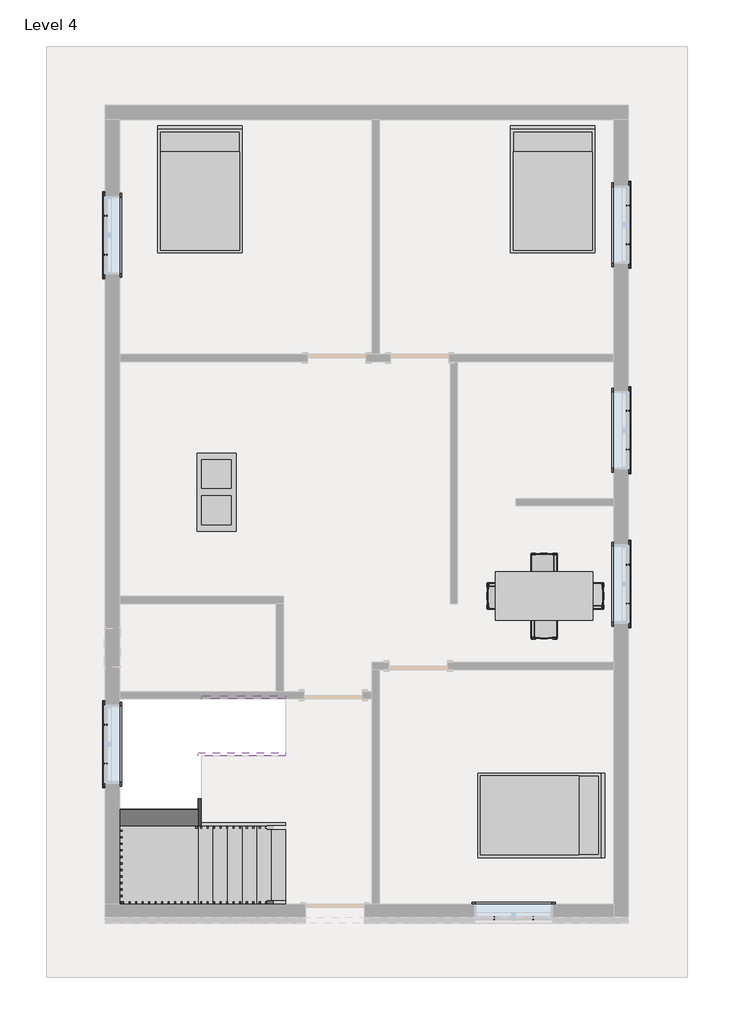
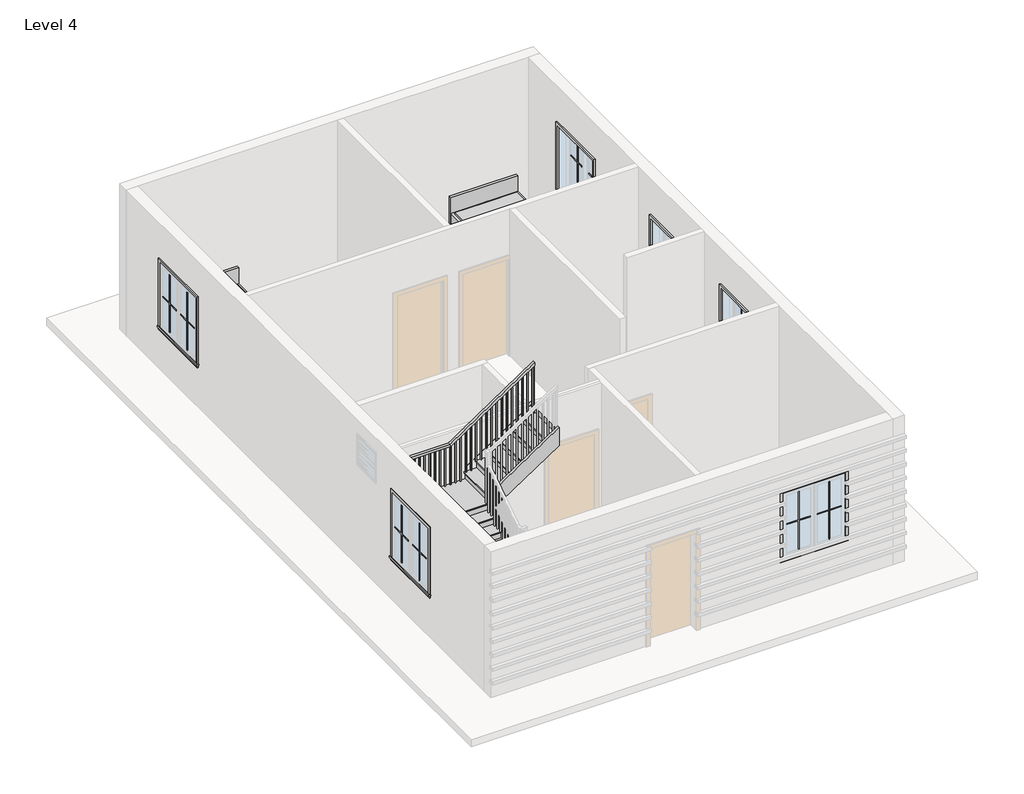
# One storey, part 3 of 3: 25 proxies, 5 members, 4 furniture elements, 1 railing, 1 stair flight.
"""IFC4 building model written with IfcOpenShell, lengths in millimetres."""

from ifc_helpers import new_model, si_unit, frame, origin, place, context, project, spatial, polyline, outline, extrude, faceted_brep, transform, mapped, element, save
from components import muntin_pattern_2x2_muntin_pattern_2x2_ba8901dc, muntin_pattern_2x2_muntin_pattern_2x2_877df4e9, trim_window_exterior_flat_with_sill_fda35bc9, trim_window_interior_flat_picture_frame_a80dbcd9, coffee_table_with_brass_mullions_11320_coffee_table_with_5962bef7, bed_17739_bed_17739_15c61121, dining_table_w_chairs_11374_0cdfc61b, stair_flight_3f57ae35

model = new_model("IFC4")

# Units and contexts
model_context = context("Model", 3, world=origin())
ifc_project = project(units=[si_unit("LENGTHUNIT", "METRE", prefix="MILLI")], contexts=[model_context])

# Site, building, storey
site = spatial("IfcSite", under=ifc_project)
building = spatial("IfcBuilding", under=site)
storey = spatial("IfcBuildingStorey", under=building, Name="Level 4", Elevation=9448.8)

# Proxies
placement = place(None, origin())
muntin_pattern_2x2_muntin_pattern_2x2_shape = muntin_pattern_2x2_muntin_pattern_2x2_ba8901dc(model_context)
element("IfcBuildingElementProxy", 1, Name="Muntin Pattern_2x2 : Muntin Pattern_2x2", ObjectType="Muntin Pattern_2x2 : Muntin Pattern_2x2", at=placement, inside=storey, context=model_context, shape_type="MappedRepresentation", body=[
    mapped(muntin_pattern_2x2_muntin_pattern_2x2_shape, transform((-5325.0867403, -4189.9051559, 10433.05), x_axis=(0.0, 1.0, 0.0), y_axis=(-1.0, 0.0, 0.0), z_axis=(0.0, 0.0, 1.0))),
])
element("IfcBuildingElementProxy", 2, Name="Muntin Pattern_2x2 : Muntin Pattern_2x2", ObjectType="Muntin Pattern_2x2 : Muntin Pattern_2x2", at=placement, inside=storey, context=model_context, shape_type="MappedRepresentation", body=[
    mapped(muntin_pattern_2x2_muntin_pattern_2x2_shape, transform((-5325.0867403, 3744.4198441, 10433.05), x_axis=(0.0, 1.0, 0.0), y_axis=(-1.0, 0.0, 0.0), z_axis=(0.0, 0.0, 1.0))),
])
element("IfcBuildingElementProxy", 3, Name="Muntin Pattern_2x2 : Muntin Pattern_2x2", ObjectType="Muntin Pattern_2x2 : Muntin Pattern_2x2", at=placement, inside=storey, context=model_context, shape_type="MappedRepresentation", body=[
    mapped(muntin_pattern_2x2_muntin_pattern_2x2_shape, transform((2821.9632597, 4512.7698441, 10433.05), x_axis=(0.0, -1.0, 0.0), y_axis=(1.0, 0.0, 0.0), z_axis=(0.0, 0.0, 1.0))),
])
element("IfcBuildingElementProxy", 4, Name="Muntin Pattern_2x2 : Muntin Pattern_2x2", ObjectType="Muntin Pattern_2x2 : Muntin Pattern_2x2", at=placement, inside=storey, context=model_context, shape_type="MappedRepresentation", body=[
    mapped(muntin_pattern_2x2_muntin_pattern_2x2_shape, transform((2821.9632597, 1312.3698441, 10433.05), x_axis=(0.0, -1.0, 0.0), y_axis=(1.0, 0.0, 0.0), z_axis=(0.0, 0.0, 1.0))),
])
element("IfcBuildingElementProxy", 5, Name="Muntin Pattern_2x2 : Muntin Pattern_2x2", ObjectType="Muntin Pattern_2x2 : Muntin Pattern_2x2", at=placement, inside=storey, context=model_context, shape_type="MappedRepresentation", body=[
    mapped(muntin_pattern_2x2_muntin_pattern_2x2_shape, transform((2821.9632597, -1087.9301559, 10433.05), x_axis=(0.0, -1.0, 0.0), y_axis=(1.0, 0.0, 0.0), z_axis=(0.0, 0.0, 1.0))),
])
element("IfcBuildingElementProxy", 6, Name="Muntin Pattern_2x2 : Muntin Pattern_2x2", ObjectType="Muntin Pattern_2x2 : Muntin Pattern_2x2", at=placement, inside=storey, context=model_context, shape_type="MappedRepresentation", body=[
    mapped(muntin_pattern_2x2_muntin_pattern_2x2_shape, transform((1344.0007597, -6601.3176559, 10433.05), x_axis=(-1.0, 0.0, 0.0), y_axis=(0.0, -1.0, 0.0), z_axis=(0.0, 0.0, 1.0))),
])
muntin_pattern_2x2_muntin_pattern_2x2_2_shape = muntin_pattern_2x2_muntin_pattern_2x2_877df4e9(model_context)
element("IfcBuildingElementProxy", 7, Name="Muntin Pattern_2x2 : Muntin Pattern_2x2", ObjectType="Muntin Pattern_2x2 : Muntin Pattern_2x2", at=placement, inside=storey, context=model_context, shape_type="MappedRepresentation", body=[
    mapped(muntin_pattern_2x2_muntin_pattern_2x2_2_shape, transform((-5325.0867403, -3583.4801559, 10433.05), x_axis=(0.0, -1.0, 0.0), y_axis=(1.0, 0.0, 0.0), z_axis=(0.0, 0.0, 1.0))),
])
element("IfcBuildingElementProxy", 8, Name="Muntin Pattern_2x2 : Muntin Pattern_2x2", ObjectType="Muntin Pattern_2x2 : Muntin Pattern_2x2", at=placement, inside=storey, context=model_context, shape_type="MappedRepresentation", body=[
    mapped(muntin_pattern_2x2_muntin_pattern_2x2_2_shape, transform((-5325.0867403, 4350.8448441, 10433.05), x_axis=(0.0, -1.0, 0.0), y_axis=(1.0, 0.0, 0.0), z_axis=(0.0, 0.0, 1.0))),
])
element("IfcBuildingElementProxy", 9, Name="Muntin Pattern_2x2 : Muntin Pattern_2x2", ObjectType="Muntin Pattern_2x2 : Muntin Pattern_2x2", at=placement, inside=storey, context=model_context, shape_type="MappedRepresentation", body=[
    mapped(muntin_pattern_2x2_muntin_pattern_2x2_2_shape, transform((2821.9632597, 3906.3448441, 10433.05), x_axis=(0.0, 1.0, 0.0), y_axis=(-1.0, 0.0, 0.0), z_axis=(0.0, 0.0, 1.0))),
])
element("IfcBuildingElementProxy", 10, Name="Muntin Pattern_2x2 : Muntin Pattern_2x2", ObjectType="Muntin Pattern_2x2 : Muntin Pattern_2x2", at=placement, inside=storey, context=model_context, shape_type="MappedRepresentation", body=[
    mapped(muntin_pattern_2x2_muntin_pattern_2x2_2_shape, transform((2821.9632597, 705.9448441, 10433.05), x_axis=(0.0, 1.0, 0.0), y_axis=(-1.0, 0.0, 0.0), z_axis=(0.0, 0.0, 1.0))),
])
element("IfcBuildingElementProxy", 11, Name="Muntin Pattern_2x2 : Muntin Pattern_2x2", ObjectType="Muntin Pattern_2x2 : Muntin Pattern_2x2", at=placement, inside=storey, context=model_context, shape_type="MappedRepresentation", body=[
    mapped(muntin_pattern_2x2_muntin_pattern_2x2_2_shape, transform((2821.9632597, -1694.3551559, 10433.05), x_axis=(0.0, 1.0, 0.0), y_axis=(-1.0, 0.0, 0.0), z_axis=(0.0, 0.0, 1.0))),
])
element("IfcBuildingElementProxy", 12, Name="Muntin Pattern_2x2 : Muntin Pattern_2x2", ObjectType="Muntin Pattern_2x2 : Muntin Pattern_2x2", at=placement, inside=storey, context=model_context, shape_type="MappedRepresentation", body=[
    mapped(muntin_pattern_2x2_muntin_pattern_2x2_2_shape, transform((737.5757597, -6601.3176559, 10433.05), x_axis=(1.0, 0.0, 0.0), y_axis=(0.0, 1.0, 0.0), z_axis=(0.0, 0.0, 1.0))),
])
trim_window_exterior_flat_with_sill_shape = trim_window_exterior_flat_with_sill_fda35bc9(model_context)
element("IfcBuildingElementProxy", 13, Name="Trim-Window-Exterior-Flat : with Sill", ObjectType="Trim-Window-Exterior-Flat : with Sill", at=placement, inside=storey, context=model_context, shape_type="MappedRepresentation", body=[
    mapped(trim_window_exterior_flat_with_sill_shape, transform((-5334.6117403, -3886.6926559, 11709.4), x_axis=(0.0, -1.0, 0.0), y_axis=(0.0, 0.0, 1.0), z_axis=(-1.0, 0.0, 0.0))),
])
element("IfcBuildingElementProxy", 14, Name="Trim-Window-Exterior-Flat : with Sill", ObjectType="Trim-Window-Exterior-Flat : with Sill", at=placement, inside=storey, context=model_context, shape_type="MappedRepresentation", body=[
    mapped(trim_window_exterior_flat_with_sill_shape, transform((-5334.6117403, 4047.6323441, 11709.4), x_axis=(0.0, -1.0, 0.0), y_axis=(0.0, 0.0, 1.0), z_axis=(-1.0, 0.0, 0.0))),
])
element("IfcBuildingElementProxy", 15, Name="Trim-Window-Exterior-Flat : with Sill", ObjectType="Trim-Window-Exterior-Flat : with Sill", at=placement, inside=storey, context=model_context, shape_type="MappedRepresentation", body=[
    mapped(trim_window_exterior_flat_with_sill_shape, transform((2831.4882597, 4209.5573441, 11709.4), x_axis=(0.0, 1.0, 0.0), y_axis=(0.0, 0.0, 1.0), z_axis=(1.0, 0.0, 0.0))),
])
element("IfcBuildingElementProxy", 16, Name="Trim-Window-Exterior-Flat : with Sill", ObjectType="Trim-Window-Exterior-Flat : with Sill", at=placement, inside=storey, context=model_context, shape_type="MappedRepresentation", body=[
    mapped(trim_window_exterior_flat_with_sill_shape, transform((2831.4882597, 1009.1573441, 11709.4), x_axis=(0.0, 1.0, 0.0), y_axis=(0.0, 0.0, 1.0), z_axis=(1.0, 0.0, 0.0))),
])
element("IfcBuildingElementProxy", 17, Name="Trim-Window-Exterior-Flat : with Sill", ObjectType="Trim-Window-Exterior-Flat : with Sill", at=placement, inside=storey, context=model_context, shape_type="MappedRepresentation", body=[
    mapped(trim_window_exterior_flat_with_sill_shape, transform((2831.4882597, -1391.1426559, 11709.4), x_axis=(0.0, 1.0, 0.0), y_axis=(0.0, 0.0, 1.0), z_axis=(1.0, 0.0, 0.0))),
])
element("IfcBuildingElementProxy", 18, Name="Trim-Window-Exterior-Flat : with Sill", ObjectType="Trim-Window-Exterior-Flat : with Sill", at=placement, inside=storey, context=model_context, shape_type="MappedRepresentation", body=[
    mapped(trim_window_exterior_flat_with_sill_shape, transform((1040.7882597, -6610.8426559, 11709.4), x_axis=(1.0, 0.0, 0.0), y_axis=(0.0, 0.0, 1.0), z_axis=(0.0, -1.0, 0.0))),
])
trim_window_interior_flat_picture_frame_shape = trim_window_interior_flat_picture_frame_a80dbcd9(model_context)
element("IfcBuildingElementProxy", 19, Name="Trim-Window-Interior-Flat : Picture Frame", ObjectType="Trim-Window-Interior-Flat : Picture Frame", at=placement, inside=storey, context=model_context, shape_type="MappedRepresentation", body=[
    mapped(trim_window_interior_flat_picture_frame_shape, transform((-5106.0117403, -3886.6926559, 11709.4), x_axis=(0.0, 1.0, 0.0), y_axis=(0.0, 0.0, 1.0), z_axis=(1.0, 0.0, 0.0))),
])
element("IfcBuildingElementProxy", 20, Name="Trim-Window-Interior-Flat : Picture Frame", ObjectType="Trim-Window-Interior-Flat : Picture Frame", at=placement, inside=storey, context=model_context, shape_type="MappedRepresentation", body=[
    mapped(trim_window_interior_flat_picture_frame_shape, transform((-5106.0117403, 4047.6323441, 11709.4), x_axis=(0.0, 1.0, 0.0), y_axis=(0.0, 0.0, 1.0), z_axis=(1.0, 0.0, 0.0))),
])
element("IfcBuildingElementProxy", 21, Name="Trim-Window-Interior-Flat : Picture Frame", ObjectType="Trim-Window-Interior-Flat : Picture Frame", at=placement, inside=storey, context=model_context, shape_type="MappedRepresentation", body=[
    mapped(trim_window_interior_flat_picture_frame_shape, transform((2602.8882597, 4209.5573441, 11709.4), x_axis=(0.0, -1.0, 0.0), y_axis=(0.0, 0.0, 1.0), z_axis=(-1.0, 0.0, 0.0))),
])
element("IfcBuildingElementProxy", 22, Name="Trim-Window-Interior-Flat : Picture Frame", ObjectType="Trim-Window-Interior-Flat : Picture Frame", at=placement, inside=storey, context=model_context, shape_type="MappedRepresentation", body=[
    mapped(trim_window_interior_flat_picture_frame_shape, transform((2602.8882597, 1009.1573441, 11709.4), x_axis=(0.0, -1.0, 0.0), y_axis=(0.0, 0.0, 1.0), z_axis=(-1.0, 0.0, 0.0))),
])
element("IfcBuildingElementProxy", 23, Name="Trim-Window-Interior-Flat : Picture Frame", ObjectType="Trim-Window-Interior-Flat : Picture Frame", at=placement, inside=storey, context=model_context, shape_type="MappedRepresentation", body=[
    mapped(trim_window_interior_flat_picture_frame_shape, transform((2602.8882597, -1391.1426559, 11709.4), x_axis=(0.0, -1.0, 0.0), y_axis=(0.0, 0.0, 1.0), z_axis=(-1.0, 0.0, 0.0))),
])
element("IfcBuildingElementProxy", 24, Name="Trim-Window-Interior-Flat : Picture Frame", ObjectType="Trim-Window-Interior-Flat : Picture Frame", at=placement, inside=storey, context=model_context, shape_type="MappedRepresentation", body=[
    mapped(trim_window_interior_flat_picture_frame_shape, transform((1040.7882597, -6382.2426559, 11709.4), x_axis=(-1.0, 0.0, 0.0), y_axis=(0.0, 0.0, 1.0), z_axis=(0.0, 1.0, 0.0))),
])
coffee_table_with_brass_mullions_11320_coffee_table_with_shape = coffee_table_with_brass_mullions_11320_coffee_table_with_5962bef7(model_context)
element("IfcBuildingElementProxy", 25, Name="coffee_table_with_brass_mullions_11320 : coffee_table_with_brass_mullions_11320", ObjectType="coffee_table_with_brass_mullions_11320 : coffee_table_with_brass_mullions_11320", at=placement, inside=storey, context=model_context, shape_type="MappedRepresentation", body=[
    mapped(coffee_table_with_brass_mullions_11320_coffee_table_with_shape, transform((-3162.9117403, 678.9573441, 9448.8), x_axis=(0.0, 1.0, 0.0), y_axis=(-1.0, 0.0, 0.0), z_axis=(0.0, 0.0, 1.0))),
])

# Furniture
bed_17739_bed_17739_shape = bed_17739_bed_17739_15c61121(model_context)
element("IfcFurniture", 26, ObjectType="Bed_17739 : Bed_17739", at=placement, inside=storey, context=model_context, shape_type="MappedRepresentation", body=[
    mapped(bed_17739_bed_17739_shape, transform((-3855.0617403, 4742.9573441, 9448.8), x_axis=(1.0, 0.0, 0.0), y_axis=(0.0, 1.0, 0.0), z_axis=(0.0, 0.0, 1.0))),
])
element("IfcFurniture", 27, ObjectType="Bed_17739 : Bed_17739", at=placement, inside=storey, context=model_context, shape_type="MappedRepresentation", body=[
    mapped(bed_17739_bed_17739_shape, transform((1650.3882597, 4742.9573441, 9448.8), x_axis=(1.0, 0.0, 0.0), y_axis=(0.0, 1.0, 0.0), z_axis=(0.0, 0.0, 1.0))),
])
element("IfcFurniture", 28, ObjectType="Bed_17739 : Bed_17739", at=placement, inside=storey, context=model_context, shape_type="MappedRepresentation", body=[
    mapped(bed_17739_bed_17739_shape, transform((1447.1882597, -4997.9426559, 9448.8), x_axis=(0.0, -1.0, 0.0), y_axis=(1.0, 0.0, 0.0), z_axis=(0.0, 0.0, 1.0))),
])
dining_table_w_chairs_11374_shape = dining_table_w_chairs_11374_0cdfc61b(model_context)
element("IfcFurniture", 29, ObjectType="Dining_Table_w_Chairs_11374", at=placement, inside=storey, context=model_context, shape_type="MappedRepresentation", body=[
    mapped(dining_table_w_chairs_11374_shape, transform((1497.0410232, -1671.6886654, 9448.8), x_axis=(1.0, 0.0, 0.0), y_axis=(0.0, 1.0, 0.0), z_axis=(0.0, 0.0, 1.0))),
])

# Members
element("IfcMember", 30, ObjectType="Stringer - 2\" Width", at=placement, inside=storey, context=model_context, shape_type="SweptSolid", body=[
    extrude(outline(polyline([(9448.8, -2515.2117403), (9666.8398409, -2515.2117403), (9920.8398409, -2896.2117403), (9920.8398409, -3445.6977546), (9448.8, -2737.6379933), (9448.8, -2515.2117403)])), frame((0.0, -6433.0426559, 0.0), z_axis=(0.0, 1.0, 0.0), x_axis=(0.0, 0.0, 1.0)), (0.0, 0.0, 1.0), 50.8),
])
element("IfcMember", 31, ObjectType="Stringer - 2\" Width", at=placement, inside=storey, context=model_context, shape_type="SweptSolid", body=[
    extrude(outline(polyline([(11688.1158313, -3277.2117403), (12196.1158313, -2515.2117403), (12562.4398409, -2515.2117403), (11688.1158313, -3826.6977546), (11688.1158313, -3277.2117403)])), frame((0.0, -3181.8426559, 0.0), z_axis=(0.0, 1.0, 0.0), x_axis=(0.0, 0.0, 1.0)), (0.0, 0.0, 1.0), 50.8),
])
element("IfcMember", 32, ObjectType="Stringer - 2\" Width", at=placement, inside=storey, context=model_context, shape_type="SweptSolid", body=[
    extrude(outline(polyline([(9448.8, -2515.2117403), (9666.8398409, -2515.2117403), (10547.3731743, -3836.0117403), (10181.0491647, -3836.0117403), (9448.8, -2737.6379933), (9448.8, -2515.2117403)])), frame((0.0, -5163.0426559, 0.0), z_axis=(0.0, 1.0, 0.0), x_axis=(0.0, 0.0, 1.0)), (0.0, 0.0, 1.0), 50.8),
])
element("IfcMember", 33, ObjectType="Stringer - 2\" Width", at=placement, inside=storey, context=model_context, shape_type="SweptSolid", body=[
    extrude(outline(polyline([(-5163.0426559, 10367.3158313), (-5163.0426559, 10733.6398409), (-4070.8426559, 11461.7731743), (-4070.8426559, 11095.4491647), (-5163.0426559, 10367.3158313)])), frame((-3886.8117403, 0.0, 0.0), z_axis=(1.0, 0.0, 0.0), x_axis=(0.0, 1.0, 0.0)), (0.0, 0.0, 1.0), 50.8),
])
element("IfcMember", 34, ObjectType="Stringer - 2\" Width", at=placement, inside=storey, context=model_context, shape_type="SweptSolid", body=[
    extrude(outline(polyline([(11648.0398409, -3886.8117403), (11281.7158313, -3886.8117403), (12196.1158313, -2515.2117403), (12562.4398409, -2515.2117403), (11648.0398409, -3886.8117403)])), frame((0.0, -4070.8426559, 0.0), z_axis=(0.0, 1.0, 0.0), x_axis=(0.0, 0.0, 1.0)), (0.0, 0.0, 1.0), 50.8),
])

# Railing
element("IfcRailing", 35, ObjectType="Handrail - Rectangular", at=placement, inside=storey, context=model_context, shape_type="SolidModel", body=[
    faceted_brep([(-2515.2117403, -6382.2426559, 10515.6), (-2515.2117403, -6382.2426559, 10454.5459984), (-2515.2117403, -6331.4426559, 10454.5459984), (-2515.2117403, -6331.4426559, 10515.6), (-4001.1117403, -6382.2426559, 11506.2), (-4016.4927427, -6382.2426559, 11455.4), (-4016.4927427, -6331.4426559, 11455.4), (-4001.1117403, -6331.4426559, 11506.2), (-5106.0117403, -6382.2426559, 11506.2), (-5106.0117403, -6382.2426559, 11455.4), (-5055.2117403, -6331.4426559, 11455.4), (-5055.2117403, -6331.4426559, 11506.2), (-5106.0117403, -5277.3426559, 11506.2), (-5106.0117403, -5261.9616535, 11455.4), (-5055.2117403, -5261.9616535, 11455.4), (-5055.2117403, -5277.3426559, 11506.2), (-5106.0117403, -4096.2426559, 12293.6), (-5106.0117403, -4080.8616535, 12242.8), (-5055.2117403, -4080.8616535, 12242.8), (-5055.2117403, -4096.2426559, 12293.6), (-5106.0117403, -3181.8426559, 12293.6), (-5106.0117403, -3181.8426559, 12242.8), (-5055.2117403, -3232.6426559, 12242.8), (-5055.2117403, -3232.6426559, 12293.6), (-4191.6117403, -3181.8426559, 12293.6), (-4176.2307379, -3181.8426559, 12242.8), (-4176.2307379, -3232.6426559, 12242.8), (-4191.6117403, -3232.6426559, 12293.6), (-2515.2117403, -3181.8426559, 13411.2), (-2515.2117403, -3232.6426559, 13411.2), (-2515.2117403, -3232.6426559, 13350.1459984), (-2515.2117403, -3181.8426559, 13350.1459984)], [[[0, 1, 2, 3]], [[1, 0, 4, 5]], [[2, 1, 5, 6]], [[3, 2, 6, 7]], [[0, 3, 7, 4]], [[5, 4, 8, 9]], [[6, 5, 9, 10]], [[7, 6, 10, 11]], [[4, 7, 11, 8]], [[9, 8, 12, 13]], [[10, 9, 13, 14]], [[11, 10, 14, 15]], [[8, 11, 15, 12]], [[13, 12, 16, 17]], [[14, 13, 17, 18]], [[15, 14, 18, 19]], [[12, 15, 19, 16]], [[17, 16, 20, 21]], [[18, 17, 21, 22]], [[19, 18, 22, 23]], [[16, 19, 23, 20]], [[21, 20, 24, 25]], [[22, 21, 25, 26]], [[23, 22, 26, 27]], [[20, 23, 27, 24]], [[28, 29, 30, 31]], [[25, 24, 28, 31]], [[26, 25, 31, 30]], [[27, 26, 30, 29]], [[24, 27, 29, 28]]]),
    extrude(outline(polyline([(13326.8626651, -2550.1367403), (12344.4, -2550.1367403), (12344.4, -2531.0867403), (13339.5626651, -2531.0867403), (13326.8626651, -2550.1367403)])), frame((0.0, -3216.7676559, 0.0), z_axis=(0.0, 1.0, 0.0), x_axis=(0.0, 0.0, 1.0)), (0.0, 0.0, 1.0), 19.05),
    extrude(outline(polyline([(13259.1293317, -2651.7367403), (12344.4, -2651.7367403), (12344.4, -2632.6867403), (13271.8293317, -2632.6867403), (13259.1293317, -2651.7367403)])), frame((0.0, -3216.7676559, 0.0), z_axis=(0.0, 1.0, 0.0), x_axis=(0.0, 0.0, 1.0)), (0.0, 0.0, 1.0), 19.05),
    extrude(outline(polyline([(13191.3959984, -2753.3367403), (12344.4, -2753.3367403), (12344.4, -2734.2867403), (13204.0959984, -2734.2867403), (13191.3959984, -2753.3367403)])), frame((0.0, -3216.7676559, 0.0), z_axis=(0.0, 1.0, 0.0), x_axis=(0.0, 0.0, 1.0)), (0.0, 0.0, 1.0), 19.05),
    extrude(outline(polyline([(13123.6626651, -2854.9367403), (12192.0, -2854.9367403), (12192.0, -2835.8867403), (13136.3626651, -2835.8867403), (13123.6626651, -2854.9367403)])), frame((0.0, -3216.7676559, 0.0), z_axis=(0.0, 1.0, 0.0), x_axis=(0.0, 0.0, 1.0)), (0.0, 0.0, 1.0), 19.05),
    extrude(outline(polyline([(13055.9293317, -2956.5367403), (12192.0, -2956.5367403), (12192.0, -2937.4867403), (13068.6293317, -2937.4867403), (13055.9293317, -2956.5367403)])), frame((0.0, -3216.7676559, 0.0), z_axis=(0.0, 1.0, 0.0), x_axis=(0.0, 0.0, 1.0)), (0.0, 0.0, 1.0), 19.05),
    extrude(outline(polyline([(12988.1959984, -3058.1367403), (12039.6, -3058.1367403), (12039.6, -3039.0867403), (13000.8959984, -3039.0867403), (12988.1959984, -3058.1367403)])), frame((0.0, -3216.7676559, 0.0), z_axis=(0.0, 1.0, 0.0), x_axis=(0.0, 0.0, 1.0)), (0.0, 0.0, 1.0), 19.05),
    extrude(outline(polyline([(12920.4626651, -3159.7367403), (12039.6, -3159.7367403), (12039.6, -3140.6867403), (12933.1626651, -3140.6867403), (12920.4626651, -3159.7367403)])), frame((0.0, -3216.7676559, 0.0), z_axis=(0.0, 1.0, 0.0), x_axis=(0.0, 0.0, 1.0)), (0.0, 0.0, 1.0), 19.05),
    extrude(outline(polyline([(12852.7293317, -3261.3367403), (11887.2, -3261.3367403), (11887.2, -3242.2867403), (12865.4293317, -3242.2867403), (12852.7293317, -3261.3367403)])), frame((0.0, -3216.7676559, 0.0), z_axis=(0.0, 1.0, 0.0), x_axis=(0.0, 0.0, 1.0)), (0.0, 0.0, 1.0), 19.05),
    extrude(outline(polyline([(12784.9959984, -3362.9367403), (11887.2, -3362.9367403), (11887.2, -3343.8867403), (12797.6959984, -3343.8867403), (12784.9959984, -3362.9367403)])), frame((0.0, -3216.7676559, 0.0), z_axis=(0.0, 1.0, 0.0), x_axis=(0.0, 0.0, 1.0)), (0.0, 0.0, 1.0), 19.05),
    extrude(outline(polyline([(12717.2626651, -3464.5367403), (11734.8, -3464.5367403), (11734.8, -3445.4867403), (12729.9626651, -3445.4867403), (12717.2626651, -3464.5367403)])), frame((0.0, -3216.7676559, 0.0), z_axis=(0.0, 1.0, 0.0), x_axis=(0.0, 0.0, 1.0)), (0.0, 0.0, 1.0), 19.05),
    extrude(outline(polyline([(12649.5293317, -3566.1367403), (11734.8, -3566.1367403), (11734.8, -3547.0867403), (12662.2293317, -3547.0867403), (12649.5293317, -3566.1367403)])), frame((0.0, -3216.7676559, 0.0), z_axis=(0.0, 1.0, 0.0), x_axis=(0.0, 0.0, 1.0)), (0.0, 0.0, 1.0), 19.05),
    extrude(outline(polyline([(12581.7959984, -3667.7367403), (11734.8, -3667.7367403), (11734.8, -3648.6867403), (12594.4959984, -3648.6867403), (12581.7959984, -3667.7367403)])), frame((0.0, -3216.7676559, 0.0), z_axis=(0.0, 1.0, 0.0), x_axis=(0.0, 0.0, 1.0)), (0.0, 0.0, 1.0), 19.05),
    extrude(outline(polyline([(12514.0626651, -3769.3367403), (11582.4, -3769.3367403), (11582.4, -3750.2867403), (12526.7626651, -3750.2867403), (12514.0626651, -3769.3367403)])), frame((0.0, -3216.7676559, 0.0), z_axis=(0.0, 1.0, 0.0), x_axis=(0.0, 0.0, 1.0)), (0.0, 0.0, 1.0), 19.05),
    extrude(outline(polyline([(12446.3293317, -3870.9367403), (11582.4, -3870.9367403), (11582.4, -3851.8867403), (12459.0293317, -3851.8867403), (12446.3293317, -3870.9367403)])), frame((0.0, -3216.7676559, 0.0), z_axis=(0.0, 1.0, 0.0), x_axis=(0.0, 0.0, 1.0)), (0.0, 0.0, 1.0), 19.05),
    extrude(outline(polyline([(12378.5959984, -3972.5367403), (11430.0, -3972.5367403), (11430.0, -3953.4867403), (12391.2959984, -3953.4867403), (12378.5959984, -3972.5367403)])), frame((0.0, -3216.7676559, 0.0), z_axis=(0.0, 1.0, 0.0), x_axis=(0.0, 0.0, 1.0)), (0.0, 0.0, 1.0), 19.05),
    extrude(outline(polyline([(12310.8626651, -4074.1367403), (11430.0, -4074.1367403), (11430.0, -4055.0867403), (12323.5626651, -4055.0867403), (12310.8626651, -4074.1367403)])), frame((0.0, -3216.7676559, 0.0), z_axis=(0.0, 1.0, 0.0), x_axis=(0.0, 0.0, 1.0)), (0.0, 0.0, 1.0), 19.05),
    extrude(outline(polyline([(12243.1293317, -4175.7367403), (11430.0, -4175.7367403), (11430.0, -4156.6867403), (12255.8293317, -4156.6867403), (12243.1293317, -4175.7367403)])), frame((0.0, -3216.7676559, 0.0), z_axis=(0.0, 1.0, 0.0), x_axis=(0.0, 0.0, 1.0)), (0.0, 0.0, 1.0), 19.05),
    extrude(outline(polyline([(-4277.3367403, -3197.7176559), (-4258.2867403, -3197.7176559), (-4258.2867403, -3216.7676559), (-4277.3367403, -3216.7676559), (-4277.3367403, -3197.7176559)])), frame((0.0, 0.0, 11430.0), z_axis=(0.0, 0.0, 1.0), x_axis=(1.0, 0.0, 0.0)), (0.0, 0.0, 1.0), 812.8),
    extrude(outline(polyline([(-4378.9367403, -3197.7176559), (-4359.8867403, -3197.7176559), (-4359.8867403, -3216.7676559), (-4378.9367403, -3216.7676559), (-4378.9367403, -3197.7176559)])), frame((0.0, 0.0, 11430.0), z_axis=(0.0, 0.0, 1.0), x_axis=(1.0, 0.0, 0.0)), (0.0, 0.0, 1.0), 812.8),
    extrude(outline(polyline([(-4480.5367403, -3197.7176559), (-4461.4867403, -3197.7176559), (-4461.4867403, -3216.7676559), (-4480.5367403, -3216.7676559), (-4480.5367403, -3197.7176559)])), frame((0.0, 0.0, 11430.0), z_axis=(0.0, 0.0, 1.0), x_axis=(1.0, 0.0, 0.0)), (0.0, 0.0, 1.0), 812.8),
    extrude(outline(polyline([(-4582.1367403, -3197.7176559), (-4563.0867403, -3197.7176559), (-4563.0867403, -3216.7676559), (-4582.1367403, -3216.7676559), (-4582.1367403, -3197.7176559)])), frame((0.0, 0.0, 11430.0), z_axis=(0.0, 0.0, 1.0), x_axis=(1.0, 0.0, 0.0)), (0.0, 0.0, 1.0), 812.8),
    extrude(outline(polyline([(-4683.7367403, -3197.7176559), (-4664.6867403, -3197.7176559), (-4664.6867403, -3216.7676559), (-4683.7367403, -3216.7676559), (-4683.7367403, -3197.7176559)])), frame((0.0, 0.0, 11430.0), z_axis=(0.0, 0.0, 1.0), x_axis=(1.0, 0.0, 0.0)), (0.0, 0.0, 1.0), 812.8),
    extrude(outline(polyline([(-4785.3367403, -3197.7176559), (-4766.2867403, -3197.7176559), (-4766.2867403, -3216.7676559), (-4785.3367403, -3216.7676559), (-4785.3367403, -3197.7176559)])), frame((0.0, 0.0, 11430.0), z_axis=(0.0, 0.0, 1.0), x_axis=(1.0, 0.0, 0.0)), (0.0, 0.0, 1.0), 812.8),
    extrude(outline(polyline([(-4886.9367403, -3197.7176559), (-4867.8867403, -3197.7176559), (-4867.8867403, -3216.7676559), (-4886.9367403, -3216.7676559), (-4886.9367403, -3197.7176559)])), frame((0.0, 0.0, 11430.0), z_axis=(0.0, 0.0, 1.0), x_axis=(1.0, 0.0, 0.0)), (0.0, 0.0, 1.0), 812.8),
    extrude(outline(polyline([(-4988.5367403, -3197.7176559), (-4969.4867403, -3197.7176559), (-4969.4867403, -3216.7676559), (-4988.5367403, -3216.7676559), (-4988.5367403, -3197.7176559)])), frame((0.0, 0.0, 11430.0), z_axis=(0.0, 0.0, 1.0), x_axis=(1.0, 0.0, 0.0)), (0.0, 0.0, 1.0), 812.8),
    extrude(outline(polyline([(-5090.1367403, -3318.3676559), (-5090.1367403, -3299.3176559), (-5071.0867403, -3299.3176559), (-5071.0867403, -3318.3676559), (-5090.1367403, -3318.3676559)])), frame((0.0, 0.0, 11430.0), z_axis=(0.0, 0.0, 1.0), x_axis=(1.0, 0.0, 0.0)), (0.0, 0.0, 1.0), 812.8),
    extrude(outline(polyline([(-5090.1367403, -3419.9676559), (-5090.1367403, -3400.9176559), (-5071.0867403, -3400.9176559), (-5071.0867403, -3419.9676559), (-5090.1367403, -3419.9676559)])), frame((0.0, 0.0, 11430.0), z_axis=(0.0, 0.0, 1.0), x_axis=(1.0, 0.0, 0.0)), (0.0, 0.0, 1.0), 812.8),
    extrude(outline(polyline([(-5090.1367403, -3521.5676559), (-5090.1367403, -3502.5176559), (-5071.0867403, -3502.5176559), (-5071.0867403, -3521.5676559), (-5090.1367403, -3521.5676559)])), frame((0.0, 0.0, 11430.0), z_axis=(0.0, 0.0, 1.0), x_axis=(1.0, 0.0, 0.0)), (0.0, 0.0, 1.0), 812.8),
    extrude(outline(polyline([(-5090.1367403, -3623.1676559), (-5090.1367403, -3604.1176559), (-5071.0867403, -3604.1176559), (-5071.0867403, -3623.1676559), (-5090.1367403, -3623.1676559)])), frame((0.0, 0.0, 11430.0), z_axis=(0.0, 0.0, 1.0), x_axis=(1.0, 0.0, 0.0)), (0.0, 0.0, 1.0), 812.8),
    extrude(outline(polyline([(-5090.1367403, -3724.7676559), (-5090.1367403, -3705.7176559), (-5071.0867403, -3705.7176559), (-5071.0867403, -3724.7676559), (-5090.1367403, -3724.7676559)])), frame((0.0, 0.0, 11430.0), z_axis=(0.0, 0.0, 1.0), x_axis=(1.0, 0.0, 0.0)), (0.0, 0.0, 1.0), 812.8),
    extrude(outline(polyline([(-5090.1367403, -3826.3676559), (-5090.1367403, -3807.3176559), (-5071.0867403, -3807.3176559), (-5071.0867403, -3826.3676559), (-5090.1367403, -3826.3676559)])), frame((0.0, 0.0, 11430.0), z_axis=(0.0, 0.0, 1.0), x_axis=(1.0, 0.0, 0.0)), (0.0, 0.0, 1.0), 812.8),
    extrude(outline(polyline([(-5090.1367403, -3927.9676559), (-5090.1367403, -3908.9176559), (-5071.0867403, -3908.9176559), (-5071.0867403, -3927.9676559), (-5090.1367403, -3927.9676559)])), frame((0.0, 0.0, 11430.0), z_axis=(0.0, 0.0, 1.0), x_axis=(1.0, 0.0, 0.0)), (0.0, 0.0, 1.0), 812.8),
    extrude(outline(polyline([(-5090.1367403, -4029.5676559), (-5090.1367403, -4010.5176559), (-5071.0867403, -4010.5176559), (-5071.0867403, -4029.5676559), (-5090.1367403, -4029.5676559)])), frame((0.0, 0.0, 11430.0), z_axis=(0.0, 0.0, 1.0), x_axis=(1.0, 0.0, 0.0)), (0.0, 0.0, 1.0), 812.8),
    extrude(outline(polyline([(-4112.1176559, 12221.9626651), (-4112.1176559, 11277.6), (-4131.1676559, 11277.6), (-4131.1676559, 12209.2626651), (-4112.1176559, 12221.9626651)])), frame((-5090.1367403, 0.0, 0.0), z_axis=(1.0, 0.0, 0.0), x_axis=(0.0, 1.0, 0.0)), (0.0, 0.0, 1.0), 19.05),
    extrude(outline(polyline([(-4213.7176559, 12154.2293317), (-4213.7176559, 11277.6), (-4232.7676559, 11277.6), (-4232.7676559, 12141.5293317), (-4213.7176559, 12154.2293317)])), frame((-5090.1367403, 0.0, 0.0), z_axis=(1.0, 0.0, 0.0), x_axis=(0.0, 1.0, 0.0)), (0.0, 0.0, 1.0), 19.05),
    extrude(outline(polyline([(-4315.3176559, 12086.4959984), (-4315.3176559, 11125.2), (-4334.3676559, 11125.2), (-4334.3676559, 12073.7959984), (-4315.3176559, 12086.4959984)])), frame((-5090.1367403, 0.0, 0.0), z_axis=(1.0, 0.0, 0.0), x_axis=(0.0, 1.0, 0.0)), (0.0, 0.0, 1.0), 19.05),
    extrude(outline(polyline([(-4416.9176559, 12018.7626651), (-4416.9176559, 11125.2), (-4435.9676559, 11125.2), (-4435.9676559, 12006.0626651), (-4416.9176559, 12018.7626651)])), frame((-5090.1367403, 0.0, 0.0), z_axis=(1.0, 0.0, 0.0), x_axis=(0.0, 1.0, 0.0)), (0.0, 0.0, 1.0), 19.05),
    extrude(outline(polyline([(-4518.5176559, 11951.0293317), (-4518.5176559, 10972.8), (-4537.5676559, 10972.8), (-4537.5676559, 11938.3293317), (-4518.5176559, 11951.0293317)])), frame((-5090.1367403, 0.0, 0.0), z_axis=(1.0, 0.0, 0.0), x_axis=(0.0, 1.0, 0.0)), (0.0, 0.0, 1.0), 19.05),
    extrude(outline(polyline([(-4620.1176559, 11883.2959984), (-4620.1176559, 10972.8), (-4639.1676559, 10972.8), (-4639.1676559, 11870.5959984), (-4620.1176559, 11883.2959984)])), frame((-5090.1367403, 0.0, 0.0), z_axis=(1.0, 0.0, 0.0), x_axis=(0.0, 1.0, 0.0)), (0.0, 0.0, 1.0), 19.05),
    extrude(outline(polyline([(-4721.7176559, 11815.5626651), (-4721.7176559, 10820.4), (-4740.7676559, 10820.4), (-4740.7676559, 11802.8626651), (-4721.7176559, 11815.5626651)])), frame((-5090.1367403, 0.0, 0.0), z_axis=(1.0, 0.0, 0.0), x_axis=(0.0, 1.0, 0.0)), (0.0, 0.0, 1.0), 19.05),
    extrude(outline(polyline([(-4823.3176559, 11747.8293317), (-4823.3176559, 10820.4), (-4842.3676559, 10820.4), (-4842.3676559, 11735.1293317), (-4823.3176559, 11747.8293317)])), frame((-5090.1367403, 0.0, 0.0), z_axis=(1.0, 0.0, 0.0), x_axis=(0.0, 1.0, 0.0)), (0.0, 0.0, 1.0), 19.05),
    extrude(outline(polyline([(-4924.9176559, 11680.0959984), (-4924.9176559, 10820.4), (-4943.9676559, 10820.4), (-4943.9676559, 11667.3959984), (-4924.9176559, 11680.0959984)])), frame((-5090.1367403, 0.0, 0.0), z_axis=(1.0, 0.0, 0.0), x_axis=(0.0, 1.0, 0.0)), (0.0, 0.0, 1.0), 19.05),
    extrude(outline(polyline([(-5026.5176559, 11612.3626651), (-5026.5176559, 10668.0), (-5045.5676559, 10668.0), (-5045.5676559, 11599.6626651), (-5026.5176559, 11612.3626651)])), frame((-5090.1367403, 0.0, 0.0), z_axis=(1.0, 0.0, 0.0), x_axis=(0.0, 1.0, 0.0)), (0.0, 0.0, 1.0), 19.05),
    extrude(outline(polyline([(-5128.1176559, 11544.6293317), (-5128.1176559, 10668.0), (-5147.1676559, 10668.0), (-5147.1676559, 11531.9293317), (-5128.1176559, 11544.6293317)])), frame((-5090.1367403, 0.0, 0.0), z_axis=(1.0, 0.0, 0.0), x_axis=(0.0, 1.0, 0.0)), (0.0, 0.0, 1.0), 19.05),
    extrude(outline(polyline([(-5229.7176559, 11476.8959984), (-5229.7176559, 10515.6), (-5248.7676559, 10515.6), (-5248.7676559, 11464.1959984), (-5229.7176559, 11476.8959984)])), frame((-5090.1367403, 0.0, 0.0), z_axis=(1.0, 0.0, 0.0), x_axis=(0.0, 1.0, 0.0)), (0.0, 0.0, 1.0), 19.05),
    extrude(outline(polyline([(-5090.1367403, -5350.3676559), (-5090.1367403, -5331.3176559), (-5071.0867403, -5331.3176559), (-5071.0867403, -5350.3676559), (-5090.1367403, -5350.3676559)])), frame((0.0, 0.0, 10515.6), z_axis=(0.0, 0.0, 1.0), x_axis=(1.0, 0.0, 0.0)), (0.0, 0.0, 1.0), 939.8),
    extrude(outline(polyline([(-5090.1367403, -5451.9676559), (-5090.1367403, -5432.9176559), (-5071.0867403, -5432.9176559), (-5071.0867403, -5451.9676559), (-5090.1367403, -5451.9676559)])), frame((0.0, 0.0, 10515.6), z_axis=(0.0, 0.0, 1.0), x_axis=(1.0, 0.0, 0.0)), (0.0, 0.0, 1.0), 939.8),
    extrude(outline(polyline([(-5090.1367403, -5553.5676559), (-5090.1367403, -5534.5176559), (-5071.0867403, -5534.5176559), (-5071.0867403, -5553.5676559), (-5090.1367403, -5553.5676559)])), frame((0.0, 0.0, 10515.6), z_axis=(0.0, 0.0, 1.0), x_axis=(1.0, 0.0, 0.0)), (0.0, 0.0, 1.0), 939.8),
    extrude(outline(polyline([(-5090.1367403, -5655.1676559), (-5090.1367403, -5636.1176559), (-5071.0867403, -5636.1176559), (-5071.0867403, -5655.1676559), (-5090.1367403, -5655.1676559)])), frame((0.0, 0.0, 10515.6), z_axis=(0.0, 0.0, 1.0), x_axis=(1.0, 0.0, 0.0)), (0.0, 0.0, 1.0), 939.8),
    extrude(outline(polyline([(-5090.1367403, -5756.7676559), (-5090.1367403, -5737.7176559), (-5071.0867403, -5737.7176559), (-5071.0867403, -5756.7676559), (-5090.1367403, -5756.7676559)])), frame((0.0, 0.0, 10515.6), z_axis=(0.0, 0.0, 1.0), x_axis=(1.0, 0.0, 0.0)), (0.0, 0.0, 1.0), 939.8),
    extrude(outline(polyline([(-5090.1367403, -5858.3676559), (-5090.1367403, -5839.3176559), (-5071.0867403, -5839.3176559), (-5071.0867403, -5858.3676559), (-5090.1367403, -5858.3676559)])), frame((0.0, 0.0, 10515.6), z_axis=(0.0, 0.0, 1.0), x_axis=(1.0, 0.0, 0.0)), (0.0, 0.0, 1.0), 939.8),
    extrude(outline(polyline([(-5090.1367403, -5959.9676559), (-5090.1367403, -5940.9176559), (-5071.0867403, -5940.9176559), (-5071.0867403, -5959.9676559), (-5090.1367403, -5959.9676559)])), frame((0.0, 0.0, 10515.6), z_axis=(0.0, 0.0, 1.0), x_axis=(1.0, 0.0, 0.0)), (0.0, 0.0, 1.0), 939.8),
    extrude(outline(polyline([(-5090.1367403, -6061.5676559), (-5090.1367403, -6042.5176559), (-5071.0867403, -6042.5176559), (-5071.0867403, -6061.5676559), (-5090.1367403, -6061.5676559)])), frame((0.0, 0.0, 10515.6), z_axis=(0.0, 0.0, 1.0), x_axis=(1.0, 0.0, 0.0)), (0.0, 0.0, 1.0), 939.8),
    extrude(outline(polyline([(-5090.1367403, -6163.1676559), (-5090.1367403, -6144.1176559), (-5071.0867403, -6144.1176559), (-5071.0867403, -6163.1676559), (-5090.1367403, -6163.1676559)])), frame((0.0, 0.0, 10515.6), z_axis=(0.0, 0.0, 1.0), x_axis=(1.0, 0.0, 0.0)), (0.0, 0.0, 1.0), 939.8),
    extrude(outline(polyline([(-5090.1367403, -6264.7676559), (-5090.1367403, -6245.7176559), (-5071.0867403, -6245.7176559), (-5071.0867403, -6264.7676559), (-5090.1367403, -6264.7676559)])), frame((0.0, 0.0, 10515.6), z_axis=(0.0, 0.0, 1.0), x_axis=(1.0, 0.0, 0.0)), (0.0, 0.0, 1.0), 939.8),
    extrude(outline(polyline([(-5045.6867403, -6366.3676559), (-5064.7367403, -6366.3676559), (-5064.7367403, -6347.3176559), (-5045.6867403, -6347.3176559), (-5045.6867403, -6366.3676559)])), frame((0.0, 0.0, 10515.6), z_axis=(0.0, 0.0, 1.0), x_axis=(1.0, 0.0, 0.0)), (0.0, 0.0, 1.0), 939.8),
    extrude(outline(polyline([(-4944.0867403, -6366.3676559), (-4963.1367403, -6366.3676559), (-4963.1367403, -6347.3176559), (-4944.0867403, -6347.3176559), (-4944.0867403, -6366.3676559)])), frame((0.0, 0.0, 10515.6), z_axis=(0.0, 0.0, 1.0), x_axis=(1.0, 0.0, 0.0)), (0.0, 0.0, 1.0), 939.8),
    extrude(outline(polyline([(-4842.4867403, -6366.3676559), (-4861.5367403, -6366.3676559), (-4861.5367403, -6347.3176559), (-4842.4867403, -6347.3176559), (-4842.4867403, -6366.3676559)])), frame((0.0, 0.0, 10515.6), z_axis=(0.0, 0.0, 1.0), x_axis=(1.0, 0.0, 0.0)), (0.0, 0.0, 1.0), 939.8),
    extrude(outline(polyline([(-4740.8867403, -6366.3676559), (-4759.9367403, -6366.3676559), (-4759.9367403, -6347.3176559), (-4740.8867403, -6347.3176559), (-4740.8867403, -6366.3676559)])), frame((0.0, 0.0, 10515.6), z_axis=(0.0, 0.0, 1.0), x_axis=(1.0, 0.0, 0.0)), (0.0, 0.0, 1.0), 939.8),
    extrude(outline(polyline([(-4639.2867403, -6366.3676559), (-4658.3367403, -6366.3676559), (-4658.3367403, -6347.3176559), (-4639.2867403, -6347.3176559), (-4639.2867403, -6366.3676559)])), frame((0.0, 0.0, 10515.6), z_axis=(0.0, 0.0, 1.0), x_axis=(1.0, 0.0, 0.0)), (0.0, 0.0, 1.0), 939.8),
    extrude(outline(polyline([(-4537.6867403, -6366.3676559), (-4556.7367403, -6366.3676559), (-4556.7367403, -6347.3176559), (-4537.6867403, -6347.3176559), (-4537.6867403, -6366.3676559)])), frame((0.0, 0.0, 10515.6), z_axis=(0.0, 0.0, 1.0), x_axis=(1.0, 0.0, 0.0)), (0.0, 0.0, 1.0), 939.8),
    extrude(outline(polyline([(-4436.0867403, -6366.3676559), (-4455.1367403, -6366.3676559), (-4455.1367403, -6347.3176559), (-4436.0867403, -6347.3176559), (-4436.0867403, -6366.3676559)])), frame((0.0, 0.0, 10515.6), z_axis=(0.0, 0.0, 1.0), x_axis=(1.0, 0.0, 0.0)), (0.0, 0.0, 1.0), 939.8),
    extrude(outline(polyline([(-4334.4867403, -6366.3676559), (-4353.5367403, -6366.3676559), (-4353.5367403, -6347.3176559), (-4334.4867403, -6347.3176559), (-4334.4867403, -6366.3676559)])), frame((0.0, 0.0, 10515.6), z_axis=(0.0, 0.0, 1.0), x_axis=(1.0, 0.0, 0.0)), (0.0, 0.0, 1.0), 939.8),
    extrude(outline(polyline([(-4232.8867403, -6366.3676559), (-4251.9367403, -6366.3676559), (-4251.9367403, -6347.3176559), (-4232.8867403, -6347.3176559), (-4232.8867403, -6366.3676559)])), frame((0.0, 0.0, 10515.6), z_axis=(0.0, 0.0, 1.0), x_axis=(1.0, 0.0, 0.0)), (0.0, 0.0, 1.0), 939.8),
    extrude(outline(polyline([(-4131.2867403, -6366.3676559), (-4150.3367403, -6366.3676559), (-4150.3367403, -6347.3176559), (-4131.2867403, -6347.3176559), (-4131.2867403, -6366.3676559)])), frame((0.0, 0.0, 10515.6), z_axis=(0.0, 0.0, 1.0), x_axis=(1.0, 0.0, 0.0)), (0.0, 0.0, 1.0), 939.8),
    extrude(outline(polyline([(-4029.6867403, -6366.3676559), (-4048.7367403, -6366.3676559), (-4048.7367403, -6347.3176559), (-4029.6867403, -6347.3176559), (-4029.6867403, -6366.3676559)])), frame((0.0, 0.0, 10515.6), z_axis=(0.0, 0.0, 1.0), x_axis=(1.0, 0.0, 0.0)), (0.0, 0.0, 1.0), 939.8),
    extrude(outline(polyline([(11409.1626651, -3947.1367403), (10515.6, -3947.1367403), (10515.6, -3928.0867403), (11396.4626651, -3928.0867403), (11409.1626651, -3947.1367403)])), frame((0.0, -6366.3676559, 0.0), z_axis=(0.0, 1.0, 0.0), x_axis=(0.0, 0.0, 1.0)), (0.0, 0.0, 1.0), 19.05),
    extrude(outline(polyline([(11341.4293317, -3845.5367403), (10363.2, -3845.5367403), (10363.2, -3826.4867403), (11328.7293317, -3826.4867403), (11341.4293317, -3845.5367403)])), frame((0.0, -6366.3676559, 0.0), z_axis=(0.0, 1.0, 0.0), x_axis=(0.0, 0.0, 1.0)), (0.0, 0.0, 1.0), 19.05),
    extrude(outline(polyline([(11273.6959984, -3743.9367403), (10363.2, -3743.9367403), (10363.2, -3724.8867403), (11260.9959984, -3724.8867403), (11273.6959984, -3743.9367403)])), frame((0.0, -6366.3676559, 0.0), z_axis=(0.0, 1.0, 0.0), x_axis=(0.0, 0.0, 1.0)), (0.0, 0.0, 1.0), 19.05),
    extrude(outline(polyline([(11205.9626651, -3642.3367403), (10210.8, -3642.3367403), (10210.8, -3623.2867403), (11193.2626651, -3623.2867403), (11205.9626651, -3642.3367403)])), frame((0.0, -6366.3676559, 0.0), z_axis=(0.0, 1.0, 0.0), x_axis=(0.0, 0.0, 1.0)), (0.0, 0.0, 1.0), 19.05),
    extrude(outline(polyline([(11138.2293317, -3540.7367403), (10210.8, -3540.7367403), (10210.8, -3521.6867403), (11125.5293317, -3521.6867403), (11138.2293317, -3540.7367403)])), frame((0.0, -6366.3676559, 0.0), z_axis=(0.0, 1.0, 0.0), x_axis=(0.0, 0.0, 1.0)), (0.0, 0.0, 1.0), 19.05),
    extrude(outline(polyline([(11070.4959984, -3439.1367403), (10210.8, -3439.1367403), (10210.8, -3420.0867403), (11057.7959984, -3420.0867403), (11070.4959984, -3439.1367403)])), frame((0.0, -6366.3676559, 0.0), z_axis=(0.0, 1.0, 0.0), x_axis=(0.0, 0.0, 1.0)), (0.0, 0.0, 1.0), 19.05),
    extrude(outline(polyline([(11002.7626651, -3337.5367403), (10058.4, -3337.5367403), (10058.4, -3318.4867403), (10990.0626651, -3318.4867403), (11002.7626651, -3337.5367403)])), frame((0.0, -6366.3676559, 0.0), z_axis=(0.0, 1.0, 0.0), x_axis=(0.0, 0.0, 1.0)), (0.0, 0.0, 1.0), 19.05),
    extrude(outline(polyline([(10935.0293317, -3235.9367403), (10058.4, -3235.9367403), (10058.4, -3216.8867403), (10922.3293317, -3216.8867403), (10935.0293317, -3235.9367403)])), frame((0.0, -6366.3676559, 0.0), z_axis=(0.0, 1.0, 0.0), x_axis=(0.0, 0.0, 1.0)), (0.0, 0.0, 1.0), 19.05),
    extrude(outline(polyline([(10867.2959984, -3134.3367403), (9906.0, -3134.3367403), (9906.0, -3115.2867403), (10854.5959984, -3115.2867403), (10867.2959984, -3134.3367403)])), frame((0.0, -6366.3676559, 0.0), z_axis=(0.0, 1.0, 0.0), x_axis=(0.0, 0.0, 1.0)), (0.0, 0.0, 1.0), 19.05),
    extrude(outline(polyline([(10799.5626651, -3032.7367403), (9906.0, -3032.7367403), (9906.0, -3013.6867403), (10786.8626651, -3013.6867403), (10799.5626651, -3032.7367403)])), frame((0.0, -6366.3676559, 0.0), z_axis=(0.0, 1.0, 0.0), x_axis=(0.0, 0.0, 1.0)), (0.0, 0.0, 1.0), 19.05),
    extrude(outline(polyline([(10731.8293317, -2931.1367403), (9753.6, -2931.1367403), (9753.6, -2912.0867403), (10719.1293317, -2912.0867403), (10731.8293317, -2931.1367403)])), frame((0.0, -6366.3676559, 0.0), z_axis=(0.0, 1.0, 0.0), x_axis=(0.0, 0.0, 1.0)), (0.0, 0.0, 1.0), 19.05),
    extrude(outline(polyline([(10664.0959984, -2829.5367403), (9753.6, -2829.5367403), (9753.6, -2810.4867403), (10651.3959984, -2810.4867403), (10664.0959984, -2829.5367403)])), frame((0.0, -6366.3676559, 0.0), z_axis=(0.0, 1.0, 0.0), x_axis=(0.0, 0.0, 1.0)), (0.0, 0.0, 1.0), 19.05),
    extrude(outline(polyline([(10596.3626651, -2727.9367403), (9601.2, -2727.9367403), (9601.2, -2708.8867403), (10583.6626651, -2708.8867403), (10596.3626651, -2727.9367403)])), frame((0.0, -6366.3676559, 0.0), z_axis=(0.0, 1.0, 0.0), x_axis=(0.0, 0.0, 1.0)), (0.0, 0.0, 1.0), 19.05),
    extrude(outline(polyline([(10528.6293317, -2626.3367403), (9601.2, -2626.3367403), (9601.2, -2607.2867403), (10515.9293317, -2607.2867403), (10528.6293317, -2626.3367403)])), frame((0.0, -6366.3676559, 0.0), z_axis=(0.0, 1.0, 0.0), x_axis=(0.0, 0.0, 1.0)), (0.0, 0.0, 1.0), 19.05),
    extrude(outline(polyline([(-5090.1367403, -3216.7676559), (-5090.1367403, -3197.7176559), (-5071.0867403, -3197.7176559), (-5071.0867403, -3216.7676559), (-5090.1367403, -3216.7676559)])), frame((0.0, 0.0, 11430.0), z_axis=(0.0, 0.0, 1.0), x_axis=(1.0, 0.0, 0.0)), (0.0, 0.0, 1.0), 812.8),
    extrude(outline(polyline([(-5071.0867403, -6366.3676559), (-5090.1367403, -6366.3676559), (-5090.1367403, -6347.3176559), (-5071.0867403, -6347.3176559), (-5071.0867403, -6366.3676559)])), frame((0.0, 0.0, 10515.6), z_axis=(0.0, 0.0, 1.0), x_axis=(1.0, 0.0, 0.0)), (0.0, 0.0, 1.0), 939.8),
    extrude(outline(polyline([(13337.4459984, -2534.2617403), (12344.4, -2534.2617403), (12344.4, -2515.2117403), (13350.1459984, -2515.2117403), (13337.4459984, -2534.2617403)])), frame((0.0, -3216.7676559, 0.0), z_axis=(0.0, 1.0, 0.0), x_axis=(0.0, 0.0, 1.0)), (0.0, 0.0, 1.0), 19.05),
    extrude(outline(polyline([(10467.2459984, -2534.2617403), (9601.2, -2534.2617403), (9601.2, -2515.2117403), (10454.5459984, -2515.2117403), (10467.2459984, -2534.2617403)])), frame((0.0, -6366.3676559, 0.0), z_axis=(0.0, 1.0, 0.0), x_axis=(0.0, 0.0, 1.0)), (0.0, 0.0, 1.0), 19.05),
])

# Stair flight
stair_flight_shape = stair_flight_3f57ae35(model_context)
element("IfcStairFlight", 36, ObjectType="2\" Tread 1\" Nosing 1/4\" Riser", at=placement, inside=storey, context=model_context, shape_type="MappedRepresentation", body=[
    mapped(stair_flight_shape, transform((0.0, 0.0, 0.0), x_axis=(1.0, 0.0, 0.0), y_axis=(0.0, 1.0, 0.0), z_axis=(0.0, 0.0, 1.0))),
])

save(model, "model.ifc")

# Revit data of these elements
# Type "Muntin Pattern_2x2 : Muntin Pattern_2x2"
#   Width [instance default] = 4' - 0"
#   Thickness = 0' - 0 1/2"
#   Height [instance default] = 4' - 0"
#   Distance = 0' - 0 3/4"
#   Interior Material [instance default] = none
#   Exterior Material [instance default] = none
#   Default Elevation = 0
# Type "Trim-Window-Exterior-Flat : with Sill"
#   Trim Width = 0' - 2 1/4"
#   Trim Thickness_Picture Frame = 0' - 1 1/4"
#   Trim Thickness_with Sill = 0' - 0 3/4"
#   Sill Thickness = 0' - 1 1/4"
#   Opening Width [instance default] = 2' - 0"
#   Opening Height [instance default] = 3' - 0"
#   Default Elevation = 4' - 0"
#   Sill = yes
#   Picture Frame = no
#   Trim Material [instance default] = none
# Type "Trim-Window-Interior-Flat : Picture Frame"
#   Trim Thickness_Picture Frame = 0' - 1 1/4"
#   Trim Width = 0' - 2 1/4"
#   Trim Thickness_with Sill = 0' - 0 3/4"
#   Sill Thickness = 0' - 1 1/4"
#   Opening Width [instance default] = 2' - 0"
#   Opening Height [instance default] = 3' - 0"
#   Default Elevation = 4' - 0"
#   Sill = no
#   Picture Frame = yes
#   Trim Material [instance default] = none
# Type "coffee_table_with_brass_mullions_11320 : coffee_table_with_brass_mullions_11320"
#   Default Elevation = 0
# Type "Bed_17739 : Bed_17739"
#   Default Elevation = 0
# Type "Dining_Table_w_Chairs_11374"
#   Default Elevation = 0
#   Assembly Code = ""
# Type "Handrail - Rectangular"
#   Assembly Code = "C2010400"
#   built-in parameter 1008612 = 0.0416667 (stored number, unit not read)
#   built-in parameter 1008611 = 0.0416667 (stored number, unit not read)
#   built-in parameter 1008609 = 0.333333 (stored number, unit not read)
#   built-in parameter 1008604 = 0.166667 (stored number, unit not read)
#   built-in parameter 1008603 = 0.166667 (stored number, unit not read)
#   Railing Height = 3' - 0"
#   built-in parameter 1008630 = 2
#   built-in parameter 1008610 = 2
#   built-in parameter 1008618 = Baluster - Square : 3/4"
# Elements 1, 2, 3, 4, 5, 6, 7, 8, 9, 10, 11, 12 (IfcBuildingElementProxy, "Muntin Pattern_2x2 : Muntin Pattern_2x2")
#   Width = 1' - 6 5/8"
#   Height = 3' - 11 1/2"
#   Interior Material = Wood - Stained
#   Exterior Material = Clad - White
#   Phase Created = New Construction
#   Materials on its faces: "Clad - White", "Wood - Stained"
# Elements 13, 14, 15, 16, 17, 18 (IfcBuildingElementProxy, "Trim-Window-Exterior-Flat : with Sill")
#   Opening Width = 4' - 0"
#   Opening Height = 4' - 5"
#   Trim Material = Clad - White
#   Phase Created = New Construction
#   Materials on its faces: "Clad - White"
# Elements 19, 20, 21, 22, 23, 24 (IfcBuildingElementProxy, "Trim-Window-Interior-Flat : Picture Frame")
#   Opening Width = 4' - 0"
#   Opening Height = 4' - 5"
#   Trim Material = Wood - Stained
#   Phase Created = New Construction
#   Materials on its faces: "Wood - Stained"
# Element 25 (IfcBuildingElementProxy, "coffee_table_with_brass_mullions_11320 : coffee_table_with_brass_mullions_11320")
#   Phase Created = New Construction
#   Materials on its faces: "Default Wall", "TABLE", "Glass", "Default"
# Elements 26, 27, 28 (IfcFurniture, "Bed_17739 : Bed_17739")
#   Phase Created = New Construction
#   Materials on its faces: "legs", "sheets", "bed frame", "Blanket"
# Element 29 (IfcFurniture, "Dining_Table_w_Chairs_11374")
#   Phase Created = New Construction
# Elements 30, 31, 32, 33, 34 (IfcMember, "Stringer - 2\" Width")
#   Phase Created = New Construction
# Element 35 (IfcRailing, "Handrail - Rectangular")
#   Phase Created = New Construction
#   Materials on its faces: "Clad - White"
# Element 36 (IfcStairFlight, "2\" Tread 1\" Nosing 1/4\" Riser")
#   Phase Created = New Construction
#   Materials on its faces: "Wood Planks"
# Materials
#   "Clad - White": class "Wood", colour RGB 242 242 238, transparency 0, Cost = 0
#   "Wood - Stained": class "Wood", colour RGB 224 178 126, transparency 0, Cost = 0
#   "Default Wall": colour RGB 128 128 128, transparency 0, Cost = 0
#   "TABLE": class "Generic", colour RGB 120 120 120, transparency 0, Cost = 0
#   "Glass": class "Glass", colour RGB 0 128 192, transparency 0.75, Description = "Soda Lime Glass", Cost = 0
#   "Default": colour RGB 127 127 127, transparency 0, Cost = 0
#   "legs": colour RGB 90 73 37, transparency 0, Cost = 0
#   "sheets": colour RGB 200 195 176, transparency 0, Cost = 0
#   "bed frame": colour RGB 90 73 37, transparency 0, Cost = 0
#   "Blanket": class "System", colour RGB 59 0 1, transparency 0, Cost = 0
#   "Wood Planks": class "Wood", colour RGB 193 160 115, transparency 0, Description = "Physical material.", Cost = 0
